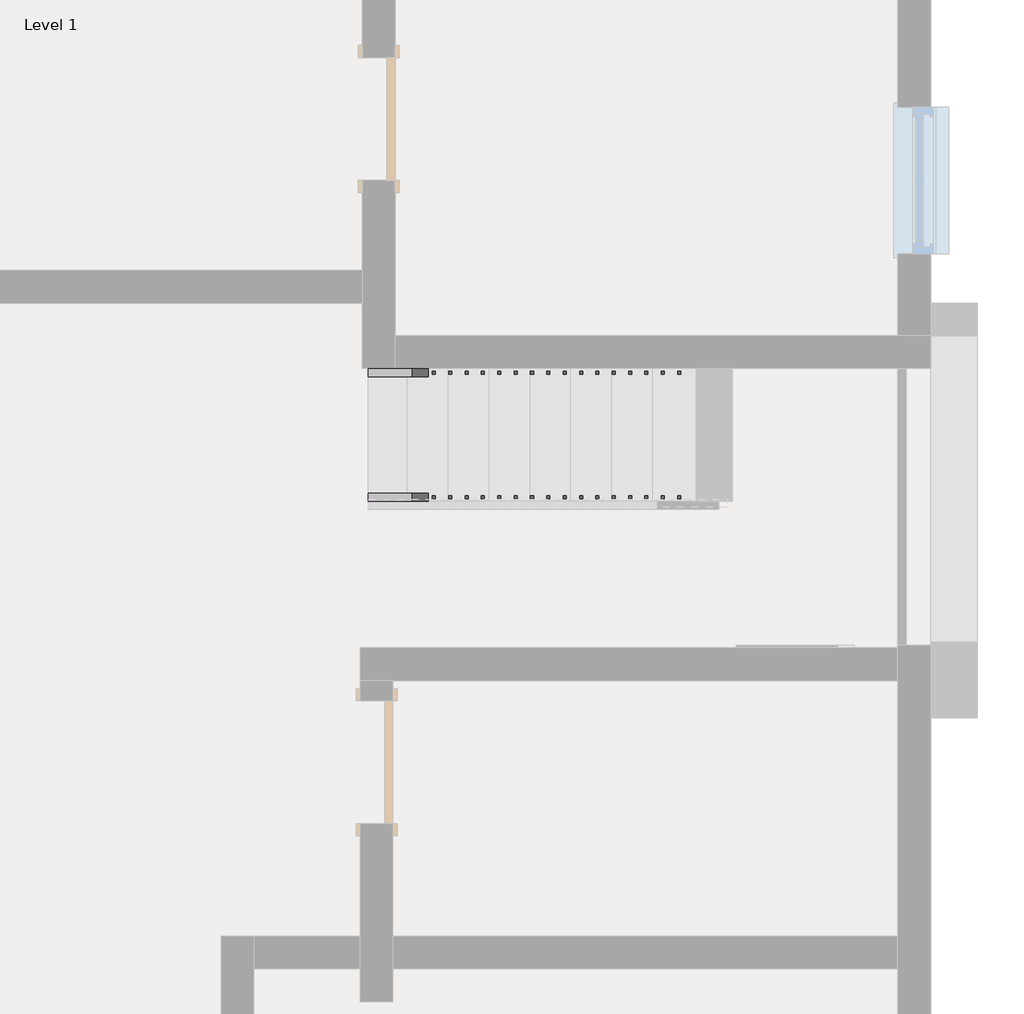
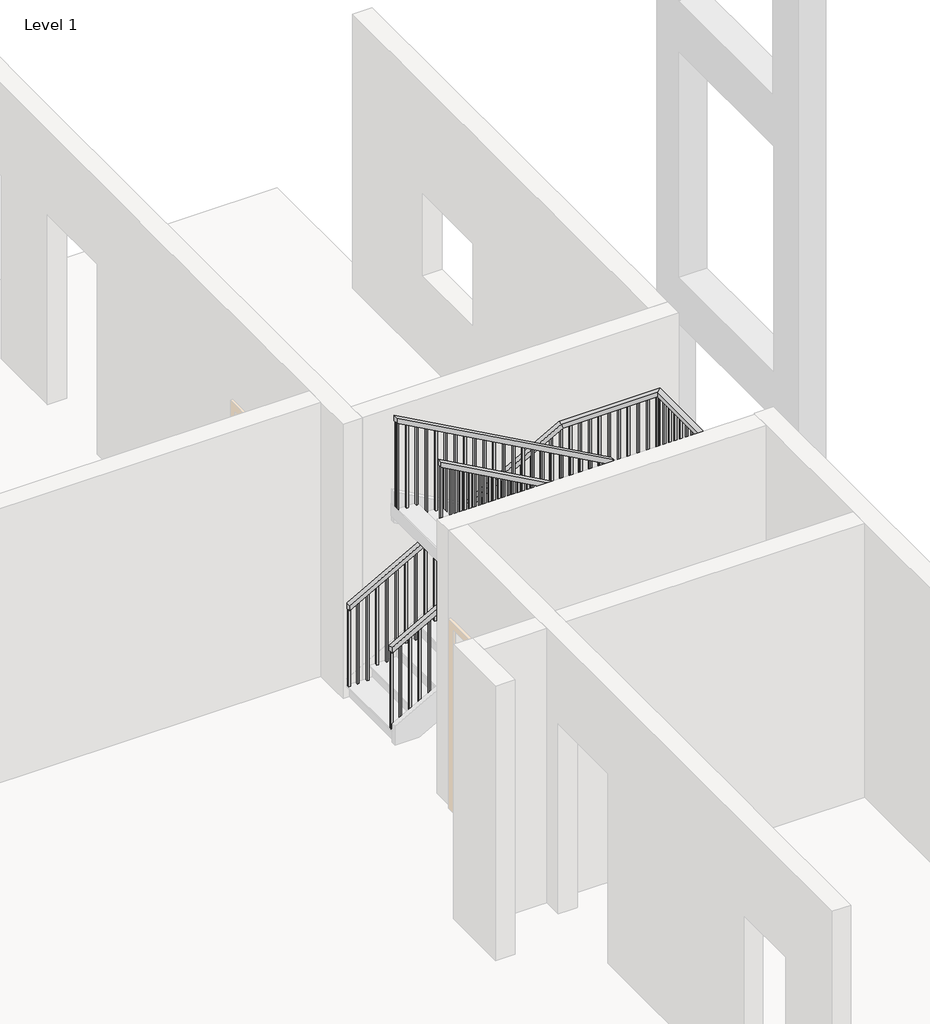
# One storey, part 3 of 4: 2 railings.
"""IFC4 building model written with IfcOpenShell, lengths in millimetres."""

from ifc_helpers import new_model, si_unit, frame, origin, place, context, project, spatial, polyline, outline, extrude, faceted_brep, element, save

model = new_model("IFC4")

# Units and contexts
model_context = context("Model", 3, world=origin())
ifc_project = project(units=[si_unit("LENGTHUNIT", "METRE", prefix="MILLI")], contexts=[model_context])

# Site, building, storey
site = spatial("IfcSite", under=ifc_project)
building = spatial("IfcBuilding", under=site)
storey = spatial("IfcBuildingStorey", under=building, Name="Level 1", Elevation=0.0)

# Railings
placement = place(None, origin())
element("IfcRailing", 1, ObjectType="Handrail - Rectangular", at=placement, inside=storey, context=model_context, shape_type="SolidModel", body=[
    faceted_brep([(1537.1941283, 231.7547293, 1051.56), (1537.1941283, 231.7547293, 993.4879132), (1537.1941283, 180.9547293, 993.4879132), (1537.1941283, 180.9547293, 1051.56), (3765.8648053, 231.7547293, 2286.0), (3765.8648053, 180.9547293, 2286.0), (3765.8648053, 180.9547293, 2227.9279132), (3765.8648053, 231.7547293, 2227.9279132)], [[[0, 1, 2, 3]], [[4, 5, 6, 7]], [[1, 0, 4, 7]], [[2, 1, 7, 6]], [[3, 2, 6, 5]], [[0, 3, 5, 4]]]),
    faceted_brep([(3816.6648053, 231.7547293, 2286.0), (3816.6648053, 231.7547293, 2235.2), (3765.8648053, 231.7547293, 2235.2), (3765.8648053, 231.7547293, 2286.0), (3816.6648053, 142.8547293, 2286.0), (3765.8648053, 142.8547293, 2286.0), (3765.8648053, 92.0547293, 2235.2), (3816.6648053, 92.0547293, 2235.2)], [[[0, 1, 2, 3]], [[4, 5, 6, 7]], [[1, 0, 4, 7]], [[2, 1, 7, 6]], [[3, 2, 6, 5]], [[0, 3, 5, 4]]]),
    faceted_brep([(3816.6648053, 142.8547293, 2286.0), (3816.6648053, 92.0547293, 2235.2), (3765.8648053, 92.0547293, 2235.2), (3765.8648053, 142.8547293, 2286.0), (3816.6648053, 142.8547293, 2395.0223516), (3765.8648053, 142.8547293, 2365.0879132), (3765.8648053, 92.0547293, 2365.0879132), (3816.6648053, 92.0547293, 2395.0223516)], [[[0, 1, 2, 3]], [[4, 5, 6, 7]], [[1, 0, 4, 7]], [[2, 1, 7, 6]], [[3, 2, 6, 5]], [[0, 3, 5, 4]]]),
    faceted_brep([(3816.6648053, 92.0547293, 2395.0223516), (3765.8648053, 92.0547293, 2365.0879132), (3765.8648053, 142.8547293, 2365.0879132), (3816.6648053, 142.8547293, 2395.0223516), (1537.1941283, 92.0547293, 3657.6), (1537.1941283, 142.8547293, 3657.6), (1537.1941283, 142.8547293, 3599.5279132), (1537.1941283, 92.0547293, 3599.5279132)], [[[0, 1, 2, 3]], [[4, 5, 6, 7]], [[1, 0, 4, 7]], [[2, 1, 7, 6]], [[3, 2, 6, 5]], [[0, 3, 5, 4]]]),
    extrude(outline(polyline([(3583.7556667, 1565.5898053), (3594.3072849, 1546.5398053), (2606.04, 1546.5398053), (2606.04, 1565.5898053), (3583.7556667, 1565.5898053)])), frame((0.0, 107.9297293, 0.0), z_axis=(0.0, 1.0, 0.0), x_axis=(0.0, 0.0, 1.0)), (0.0, 0.0, 1.0), 19.05),
    extrude(outline(polyline([(3527.4803699, 1667.1898053), (3538.031988, 1648.1398053), (2606.04, 1648.1398053), (2606.04, 1667.1898053), (3527.4803699, 1667.1898053)])), frame((0.0, 107.9297293, 0.0), z_axis=(0.0, 1.0, 0.0), x_axis=(0.0, 0.0, 1.0)), (0.0, 0.0, 1.0), 19.05),
    extrude(outline(polyline([(3471.1609284, 1768.7898053), (3481.7125466, 1749.7398053), (2606.04, 1749.7398053), (2606.04, 1768.7898053), (3471.1609284, 1768.7898053)])), frame((0.0, 107.9297293, 0.0), z_axis=(0.0, 1.0, 0.0), x_axis=(0.0, 0.0, 1.0)), (0.0, 0.0, 1.0), 19.05),
    extrude(outline(polyline([(3414.9297761, 1870.3898053), (3425.4813943, 1851.3398053), (2468.88, 1851.3398053), (2468.88, 1870.3898053), (3414.9297761, 1870.3898053)])), frame((0.0, 107.9297293, 0.0), z_axis=(0.0, 1.0, 0.0), x_axis=(0.0, 0.0, 1.0)), (0.0, 0.0, 1.0), 19.05),
    extrude(outline(polyline([(3358.6544792, 1971.9898053), (3369.2060974, 1952.9398053), (2468.88, 1952.9398053), (2468.88, 1971.9898053), (3358.6544792, 1971.9898053)])), frame((0.0, 107.9297293, 0.0), z_axis=(0.0, 1.0, 0.0), x_axis=(0.0, 0.0, 1.0)), (0.0, 0.0, 1.0), 19.05),
    extrude(outline(polyline([(3302.3791823, 2073.5898053), (3312.9308005, 2054.5398053), (2331.72, 2054.5398053), (2331.72, 2073.5898053), (3302.3791823, 2073.5898053)])), frame((0.0, 107.9297293, 0.0), z_axis=(0.0, 1.0, 0.0), x_axis=(0.0, 0.0, 1.0)), (0.0, 0.0, 1.0), 19.05),
    extrude(outline(polyline([(3246.1038855, 2175.1898053), (3256.6555036, 2156.1398053), (2331.72, 2156.1398053), (2331.72, 2175.1898053), (3246.1038855, 2175.1898053)])), frame((0.0, 107.9297293, 0.0), z_axis=(0.0, 1.0, 0.0), x_axis=(0.0, 0.0, 1.0)), (0.0, 0.0, 1.0), 19.05),
    extrude(outline(polyline([(3189.8285886, 2276.7898053), (3200.3802067, 2257.7398053), (2331.72, 2257.7398053), (2331.72, 2276.7898053), (3189.8285886, 2276.7898053)])), frame((0.0, 107.9297293, 0.0), z_axis=(0.0, 1.0, 0.0), x_axis=(0.0, 0.0, 1.0)), (0.0, 0.0, 1.0), 19.05),
    extrude(outline(polyline([(3133.5532917, 2378.3898053), (3144.1049099, 2359.3398053), (2194.56, 2359.3398053), (2194.56, 2378.3898053), (3133.5532917, 2378.3898053)])), frame((0.0, 107.9297293, 0.0), z_axis=(0.0, 1.0, 0.0), x_axis=(0.0, 0.0, 1.0)), (0.0, 0.0, 1.0), 19.05),
    extrude(outline(polyline([(3077.2779948, 2479.9898053), (3087.829613, 2460.9398053), (2194.56, 2460.9398053), (2194.56, 2479.9898053), (3077.2779948, 2479.9898053)])), frame((0.0, 107.9297293, 0.0), z_axis=(0.0, 1.0, 0.0), x_axis=(0.0, 0.0, 1.0)), (0.0, 0.0, 1.0), 19.05),
    extrude(outline(polyline([(3021.0026979, 2581.5898053), (3031.5543161, 2562.5398053), (2057.4, 2562.5398053), (2057.4, 2581.5898053), (3021.0026979, 2581.5898053)])), frame((0.0, 107.9297293, 0.0), z_axis=(0.0, 1.0, 0.0), x_axis=(0.0, 0.0, 1.0)), (0.0, 0.0, 1.0), 19.05),
    extrude(outline(polyline([(2964.727401, 2683.1898053), (2975.2790192, 2664.1398053), (2057.4, 2664.1398053), (2057.4, 2683.1898053), (2964.727401, 2683.1898053)])), frame((0.0, 107.9297293, 0.0), z_axis=(0.0, 1.0, 0.0), x_axis=(0.0, 0.0, 1.0)), (0.0, 0.0, 1.0), 19.05),
    extrude(outline(polyline([(2908.4962488, 2784.7898053), (2919.0478669, 2765.7398053), (2057.4, 2765.7398053), (2057.4, 2784.7898053), (2908.4962488, 2784.7898053)])), frame((0.0, 107.9297293, 0.0), z_axis=(0.0, 1.0, 0.0), x_axis=(0.0, 0.0, 1.0)), (0.0, 0.0, 1.0), 19.05),
    extrude(outline(polyline([(2852.2209519, 2886.3898053), (2862.77257, 2867.3398053), (1920.24, 2867.3398053), (1920.24, 2886.3898053), (2852.2209519, 2886.3898053)])), frame((0.0, 107.9297293, 0.0), z_axis=(0.0, 1.0, 0.0), x_axis=(0.0, 0.0, 1.0)), (0.0, 0.0, 1.0), 19.05),
    extrude(outline(polyline([(2795.945655, 2987.9898053), (2806.4972732, 2968.9398053), (1920.24, 2968.9398053), (1920.24, 2987.9898053), (2795.945655, 2987.9898053)])), frame((0.0, 107.9297293, 0.0), z_axis=(0.0, 1.0, 0.0), x_axis=(0.0, 0.0, 1.0)), (0.0, 0.0, 1.0), 19.05),
    extrude(outline(polyline([(2739.6703581, 3089.5898053), (2750.2219763, 3070.5398053), (1783.08, 3070.5398053), (1783.08, 3089.5898053), (2739.6703581, 3089.5898053)])), frame((0.0, 107.9297293, 0.0), z_axis=(0.0, 1.0, 0.0), x_axis=(0.0, 0.0, 1.0)), (0.0, 0.0, 1.0), 19.05),
    extrude(outline(polyline([(2683.3950612, 3191.1898053), (2693.9466794, 3172.1398053), (1783.08, 3172.1398053), (1783.08, 3191.1898053), (2683.3950612, 3191.1898053)])), frame((0.0, 107.9297293, 0.0), z_axis=(0.0, 1.0, 0.0), x_axis=(0.0, 0.0, 1.0)), (0.0, 0.0, 1.0), 19.05),
    extrude(outline(polyline([(2627.1197643, 3292.7898053), (2637.6713825, 3273.7398053), (1783.08, 3273.7398053), (1783.08, 3292.7898053), (2627.1197643, 3292.7898053)])), frame((0.0, 107.9297293, 0.0), z_axis=(0.0, 1.0, 0.0), x_axis=(0.0, 0.0, 1.0)), (0.0, 0.0, 1.0), 19.05),
    extrude(outline(polyline([(2570.8444675, 3394.3898053), (2581.3960856, 3375.3398053), (1645.92, 3375.3398053), (1645.92, 3394.3898053), (2570.8444675, 3394.3898053)])), frame((0.0, 107.9297293, 0.0), z_axis=(0.0, 1.0, 0.0), x_axis=(0.0, 0.0, 1.0)), (0.0, 0.0, 1.0), 19.05),
    extrude(outline(polyline([(2514.5691706, 3495.9898053), (2525.1207888, 3476.9398053), (1645.92, 3476.9398053), (1645.92, 3495.9898053), (2514.5691706, 3495.9898053)])), frame((0.0, 107.9297293, 0.0), z_axis=(0.0, 1.0, 0.0), x_axis=(0.0, 0.0, 1.0)), (0.0, 0.0, 1.0), 19.05),
    extrude(outline(polyline([(2458.2938737, 3597.5898053), (2468.8454919, 3578.5398053), (1508.76, 3578.5398053), (1508.76, 3597.5898053), (2458.2938737, 3597.5898053)])), frame((0.0, 107.9297293, 0.0), z_axis=(0.0, 1.0, 0.0), x_axis=(0.0, 0.0, 1.0)), (0.0, 0.0, 1.0), 19.05),
    extrude(outline(polyline([(2402.0185768, 3699.1898053), (2412.570195, 3680.1398053), (1508.76, 3680.1398053), (1508.76, 3699.1898053), (2402.0185768, 3699.1898053)])), frame((0.0, 107.9297293, 0.0), z_axis=(0.0, 1.0, 0.0), x_axis=(0.0, 0.0, 1.0)), (0.0, 0.0, 1.0), 19.05),
    extrude(outline(polyline([(2236.8202537, 3781.9191283), (2226.2686355, 3762.8691283), (1371.6, 3762.8691283), (1371.6, 3781.9191283), (2236.8202537, 3781.9191283)])), frame((0.0, 196.8297293, 0.0), z_axis=(0.0, 1.0, 0.0), x_axis=(0.0, 0.0, 1.0)), (0.0, 0.0, 1.0), 19.05),
    extrude(outline(polyline([(2180.5449568, 3680.3191283), (2169.9933387, 3661.2691283), (1234.44, 3661.2691283), (1234.44, 3680.3191283), (2180.5449568, 3680.3191283)])), frame((0.0, 196.8297293, 0.0), z_axis=(0.0, 1.0, 0.0), x_axis=(0.0, 0.0, 1.0)), (0.0, 0.0, 1.0), 19.05),
    extrude(outline(polyline([(2124.26966, 3578.7191283), (2113.7180418, 3559.6691283), (1234.44, 3559.6691283), (1234.44, 3578.7191283), (2124.26966, 3578.7191283)])), frame((0.0, 196.8297293, 0.0), z_axis=(0.0, 1.0, 0.0), x_axis=(0.0, 0.0, 1.0)), (0.0, 0.0, 1.0), 19.05),
    extrude(outline(polyline([(2067.9943631, 3477.1191283), (2057.4427449, 3458.0691283), (1097.28, 3458.0691283), (1097.28, 3477.1191283), (2067.9943631, 3477.1191283)])), frame((0.0, 196.8297293, 0.0), z_axis=(0.0, 1.0, 0.0), x_axis=(0.0, 0.0, 1.0)), (0.0, 0.0, 1.0), 19.05),
    extrude(outline(polyline([(2011.7190662, 3375.5191283), (2001.167448, 3356.4691283), (1097.28, 3356.4691283), (1097.28, 3375.5191283), (2011.7190662, 3375.5191283)])), frame((0.0, 196.8297293, 0.0), z_axis=(0.0, 1.0, 0.0), x_axis=(0.0, 0.0, 1.0)), (0.0, 0.0, 1.0), 19.05),
    extrude(outline(polyline([(1955.4437693, 3273.9191283), (1944.8921511, 3254.8691283), (960.12, 3254.8691283), (960.12, 3273.9191283), (1955.4437693, 3273.9191283)])), frame((0.0, 196.8297293, 0.0), z_axis=(0.0, 1.0, 0.0), x_axis=(0.0, 0.0, 1.0)), (0.0, 0.0, 1.0), 19.05),
    extrude(outline(polyline([(1899.1684724, 3172.3191283), (1888.6168543, 3153.2691283), (960.12, 3153.2691283), (960.12, 3172.3191283), (1899.1684724, 3172.3191283)])), frame((0.0, 196.8297293, 0.0), z_axis=(0.0, 1.0, 0.0), x_axis=(0.0, 0.0, 1.0)), (0.0, 0.0, 1.0), 19.05),
    extrude(outline(polyline([(1842.8931755, 3070.7191283), (1832.3415574, 3051.6691283), (960.12, 3051.6691283), (960.12, 3070.7191283), (1842.8931755, 3070.7191283)])), frame((0.0, 196.8297293, 0.0), z_axis=(0.0, 1.0, 0.0), x_axis=(0.0, 0.0, 1.0)), (0.0, 0.0, 1.0), 19.05),
    extrude(outline(polyline([(1786.6178787, 2969.1191283), (1776.0662605, 2950.0691283), (822.96, 2950.0691283), (822.96, 2969.1191283), (1786.6178787, 2969.1191283)])), frame((0.0, 196.8297293, 0.0), z_axis=(0.0, 1.0, 0.0), x_axis=(0.0, 0.0, 1.0)), (0.0, 0.0, 1.0), 19.05),
    extrude(outline(polyline([(1730.3425818, 2867.5191283), (1719.7909636, 2848.4691283), (822.96, 2848.4691283), (822.96, 2867.5191283), (1730.3425818, 2867.5191283)])), frame((0.0, 196.8297293, 0.0), z_axis=(0.0, 1.0, 0.0), x_axis=(0.0, 0.0, 1.0)), (0.0, 0.0, 1.0), 19.05),
    extrude(outline(polyline([(1674.0672849, 2765.9191283), (1663.5156667, 2746.8691283), (685.8, 2746.8691283), (685.8, 2765.9191283), (1674.0672849, 2765.9191283)])), frame((0.0, 196.8297293, 0.0), z_axis=(0.0, 1.0, 0.0), x_axis=(0.0, 0.0, 1.0)), (0.0, 0.0, 1.0), 19.05),
    extrude(outline(polyline([(1617.791988, 2664.3191283), (1607.2403699, 2645.2691283), (685.8, 2645.2691283), (685.8, 2664.3191283), (1617.791988, 2664.3191283)])), frame((0.0, 196.8297293, 0.0), z_axis=(0.0, 1.0, 0.0), x_axis=(0.0, 0.0, 1.0)), (0.0, 0.0, 1.0), 19.05),
    extrude(outline(polyline([(1561.4725466, 2562.7191283), (1550.9209284, 2543.6691283), (685.8, 2543.6691283), (685.8, 2562.7191283), (1561.4725466, 2562.7191283)])), frame((0.0, 196.8297293, 0.0), z_axis=(0.0, 1.0, 0.0), x_axis=(0.0, 0.0, 1.0)), (0.0, 0.0, 1.0), 19.05),
    extrude(outline(polyline([(1505.2413943, 2461.1191283), (1494.6897761, 2442.0691283), (548.64, 2442.0691283), (548.64, 2461.1191283), (1505.2413943, 2461.1191283)])), frame((0.0, 196.8297293, 0.0), z_axis=(0.0, 1.0, 0.0), x_axis=(0.0, 0.0, 1.0)), (0.0, 0.0, 1.0), 19.05),
    extrude(outline(polyline([(1448.9660974, 2359.5191283), (1438.4144792, 2340.4691283), (548.64, 2340.4691283), (548.64, 2359.5191283), (1448.9660974, 2359.5191283)])), frame((0.0, 196.8297293, 0.0), z_axis=(0.0, 1.0, 0.0), x_axis=(0.0, 0.0, 1.0)), (0.0, 0.0, 1.0), 19.05),
    extrude(outline(polyline([(1392.6908005, 2257.9191283), (1382.1391823, 2238.8691283), (411.48, 2238.8691283), (411.48, 2257.9191283), (1392.6908005, 2257.9191283)])), frame((0.0, 196.8297293, 0.0), z_axis=(0.0, 1.0, 0.0), x_axis=(0.0, 0.0, 1.0)), (0.0, 0.0, 1.0), 19.05),
    extrude(outline(polyline([(1336.4155036, 2156.3191283), (1325.8638855, 2137.2691283), (411.48, 2137.2691283), (411.48, 2156.3191283), (1336.4155036, 2156.3191283)])), frame((0.0, 196.8297293, 0.0), z_axis=(0.0, 1.0, 0.0), x_axis=(0.0, 0.0, 1.0)), (0.0, 0.0, 1.0), 19.05),
    extrude(outline(polyline([(1280.1402067, 2054.7191283), (1269.5885886, 2035.6691283), (411.48, 2035.6691283), (411.48, 2054.7191283), (1280.1402067, 2054.7191283)])), frame((0.0, 196.8297293, 0.0), z_axis=(0.0, 1.0, 0.0), x_axis=(0.0, 0.0, 1.0)), (0.0, 0.0, 1.0), 19.05),
    extrude(outline(polyline([(1223.8649099, 1953.1191283), (1213.3132917, 1934.0691283), (274.32, 1934.0691283), (274.32, 1953.1191283), (1223.8649099, 1953.1191283)])), frame((0.0, 196.8297293, 0.0), z_axis=(0.0, 1.0, 0.0), x_axis=(0.0, 0.0, 1.0)), (0.0, 0.0, 1.0), 19.05),
    extrude(outline(polyline([(1167.589613, 1851.5191283), (1157.0379948, 1832.4691283), (274.32, 1832.4691283), (274.32, 1851.5191283), (1167.589613, 1851.5191283)])), frame((0.0, 196.8297293, 0.0), z_axis=(0.0, 1.0, 0.0), x_axis=(0.0, 0.0, 1.0)), (0.0, 0.0, 1.0), 19.05),
    extrude(outline(polyline([(1111.3143161, 1749.9191283), (1100.7626979, 1730.8691283), (137.16, 1730.8691283), (137.16, 1749.9191283), (1111.3143161, 1749.9191283)])), frame((0.0, 196.8297293, 0.0), z_axis=(0.0, 1.0, 0.0), x_axis=(0.0, 0.0, 1.0)), (0.0, 0.0, 1.0), 19.05),
    extrude(outline(polyline([(1055.0390192, 1648.3191283), (1044.487401, 1629.2691283), (137.16, 1629.2691283), (137.16, 1648.3191283), (1055.0390192, 1648.3191283)])), frame((0.0, 196.8297293, 0.0), z_axis=(0.0, 1.0, 0.0), x_axis=(0.0, 0.0, 1.0)), (0.0, 0.0, 1.0), 19.05),
    extrude(outline(polyline([(3781.7398053, 126.9797293), (3800.7898053, 126.9797293), (3800.7898053, 107.9297293), (3781.7398053, 107.9297293), (3781.7398053, 126.9797293)])), frame((0.0, 0.0, 1371.6), z_axis=(0.0, 0.0, 1.0), x_axis=(1.0, 0.0, 0.0)), (0.0, 0.0, 1.0), 863.6),
    extrude(outline(polyline([(2247.2725466, 3800.7898053), (2236.7209284, 3781.7398053), (1371.6, 3781.7398053), (1371.6, 3800.7898053), (2247.2725466, 3800.7898053)])), frame((0.0, 196.8297293, 0.0), z_axis=(0.0, 1.0, 0.0), x_axis=(0.0, 0.0, 1.0)), (0.0, 0.0, 1.0), 19.05),
    extrude(outline(polyline([(3588.9762951, 1556.2441283), (3599.5279132, 1537.1941283), (2606.04, 1537.1941283), (2606.04, 1556.2441283), (3588.9762951, 1556.2441283)])), frame((0.0, 107.9297293, 0.0), z_axis=(0.0, 1.0, 0.0), x_axis=(0.0, 0.0, 1.0)), (0.0, 0.0, 1.0), 19.05),
    extrude(outline(polyline([(1004.0395314, 1556.2441283), (993.4879132, 1537.1941283), (137.16, 1537.1941283), (137.16, 1556.2441283), (1004.0395314, 1556.2441283)])), frame((0.0, 196.8297293, 0.0), z_axis=(0.0, 1.0, 0.0), x_axis=(0.0, 0.0, 1.0)), (0.0, 0.0, 1.0), 19.05),
])
element("IfcRailing", 2, ObjectType="Handrail - Rectangular", at=placement, inside=storey, context=model_context, shape_type="SolidModel", body=[
    faceted_brep([(1537.1941283, 1006.4547293, 1051.56), (1537.1941283, 1006.4547293, 993.4879132), (1537.1941283, 955.6547293, 993.4879132), (1537.1941283, 955.6547293, 1051.56), (3765.8648053, 1006.4547293, 2286.0), (3778.9939056, 1006.4547293, 2235.2), (3778.9939056, 955.6547293, 2235.2), (3765.8648053, 955.6547293, 2286.0), (4826.4941283, 1006.4547293, 2286.0), (4826.4941283, 1006.4547293, 2235.2), (4775.6941283, 955.6547293, 2235.2), (4775.6941283, 955.6547293, 2286.0), (4826.4941283, -714.2964201, 2286.0), (4826.4941283, -714.2964201, 2235.2), (4775.6941283, -663.4964201, 2235.2), (4775.6941283, -663.4964201, 2286.0), (4013.4948805, -714.2964201, 2286.0), (4000.3657803, -714.2964201, 2235.2), (4000.3657803, -663.4964201, 2235.2), (4013.4948805, -663.4964201, 2286.0), (1537.1941283, -714.2964201, 3657.6), (1537.1941283, -663.4964201, 3657.6), (1537.1941283, -663.4964201, 3599.5279132), (1537.1941283, -714.2964201, 3599.5279132)], [[[0, 1, 2, 3]], [[1, 0, 4, 5]], [[2, 1, 5, 6]], [[3, 2, 6, 7]], [[0, 3, 7, 4]], [[5, 4, 8, 9]], [[6, 5, 9, 10]], [[7, 6, 10, 11]], [[4, 7, 11, 8]], [[9, 8, 12, 13]], [[10, 9, 13, 14]], [[11, 10, 14, 15]], [[8, 11, 15, 12]], [[13, 12, 16, 17]], [[14, 13, 17, 18]], [[15, 14, 18, 19]], [[12, 15, 19, 16]], [[20, 21, 22, 23]], [[17, 16, 20, 23]], [[18, 17, 23, 22]], [[19, 18, 22, 21]], [[16, 19, 21, 20]]]),
    extrude(outline(polyline([(3597.7693102, 1540.3691283), (2606.04, 1540.3691283), (2606.04, 1559.4191283), (3587.2176921, 1559.4191283), (3597.7693102, 1540.3691283)])), frame((0.0, -698.4214201, 0.0), z_axis=(0.0, 1.0, 0.0), x_axis=(0.0, 0.0, 1.0)), (0.0, 0.0, 1.0), 19.05),
    extrude(outline(polyline([(3541.4940133, 1641.9691283), (2606.04, 1641.9691283), (2606.04, 1661.0191283), (3530.9423952, 1661.0191283), (3541.4940133, 1641.9691283)])), frame((0.0, -698.4214201, 0.0), z_axis=(0.0, 1.0, 0.0), x_axis=(0.0, 0.0, 1.0)), (0.0, 0.0, 1.0), 19.05),
    extrude(outline(polyline([(3485.2187165, 1743.5691283), (2606.04, 1743.5691283), (2606.04, 1762.6191283), (3474.6670983, 1762.6191283), (3485.2187165, 1743.5691283)])), frame((0.0, -698.4214201, 0.0), z_axis=(0.0, 1.0, 0.0), x_axis=(0.0, 0.0, 1.0)), (0.0, 0.0, 1.0), 19.05),
    extrude(outline(polyline([(3428.9434196, 1845.1691283), (2468.88, 1845.1691283), (2468.88, 1864.2191283), (3418.3918014, 1864.2191283), (3428.9434196, 1845.1691283)])), frame((0.0, -698.4214201, 0.0), z_axis=(0.0, 1.0, 0.0), x_axis=(0.0, 0.0, 1.0)), (0.0, 0.0, 1.0), 19.05),
    extrude(outline(polyline([(3372.6681227, 1946.7691283), (2468.88, 1946.7691283), (2468.88, 1965.8191283), (3362.1165045, 1965.8191283), (3372.6681227, 1946.7691283)])), frame((0.0, -698.4214201, 0.0), z_axis=(0.0, 1.0, 0.0), x_axis=(0.0, 0.0, 1.0)), (0.0, 0.0, 1.0), 19.05),
    extrude(outline(polyline([(3316.3928258, 2048.3691283), (2331.72, 2048.3691283), (2331.72, 2067.4191283), (3305.8412076, 2067.4191283), (3316.3928258, 2048.3691283)])), frame((0.0, -698.4214201, 0.0), z_axis=(0.0, 1.0, 0.0), x_axis=(0.0, 0.0, 1.0)), (0.0, 0.0, 1.0), 19.05),
    extrude(outline(polyline([(3260.1175289, 2149.9691283), (2331.72, 2149.9691283), (2331.72, 2169.0191283), (3249.5659108, 2169.0191283), (3260.1175289, 2149.9691283)])), frame((0.0, -698.4214201, 0.0), z_axis=(0.0, 1.0, 0.0), x_axis=(0.0, 0.0, 1.0)), (0.0, 0.0, 1.0), 19.05),
    extrude(outline(polyline([(3203.8422321, 2251.5691283), (2331.72, 2251.5691283), (2331.72, 2270.6191283), (3193.2906139, 2270.6191283), (3203.8422321, 2251.5691283)])), frame((0.0, -698.4214201, 0.0), z_axis=(0.0, 1.0, 0.0), x_axis=(0.0, 0.0, 1.0)), (0.0, 0.0, 1.0), 19.05),
    extrude(outline(polyline([(3147.5669352, 2353.1691283), (2194.56, 2353.1691283), (2194.56, 2372.2191283), (3137.015317, 2372.2191283), (3147.5669352, 2353.1691283)])), frame((0.0, -698.4214201, 0.0), z_axis=(0.0, 1.0, 0.0), x_axis=(0.0, 0.0, 1.0)), (0.0, 0.0, 1.0), 19.05),
    extrude(outline(polyline([(3091.2916383, 2454.7691283), (2194.56, 2454.7691283), (2194.56, 2473.8191283), (3080.7400201, 2473.8191283), (3091.2916383, 2454.7691283)])), frame((0.0, -698.4214201, 0.0), z_axis=(0.0, 1.0, 0.0), x_axis=(0.0, 0.0, 1.0)), (0.0, 0.0, 1.0), 19.05),
    extrude(outline(polyline([(3035.0163414, 2556.3691283), (2057.4, 2556.3691283), (2057.4, 2575.4191283), (3024.4647232, 2575.4191283), (3035.0163414, 2556.3691283)])), frame((0.0, -698.4214201, 0.0), z_axis=(0.0, 1.0, 0.0), x_axis=(0.0, 0.0, 1.0)), (0.0, 0.0, 1.0), 19.05),
    extrude(outline(polyline([(2978.7410445, 2657.9691283), (2057.4, 2657.9691283), (2057.4, 2677.0191283), (2968.1894264, 2677.0191283), (2978.7410445, 2657.9691283)])), frame((0.0, -698.4214201, 0.0), z_axis=(0.0, 1.0, 0.0), x_axis=(0.0, 0.0, 1.0)), (0.0, 0.0, 1.0), 19.05),
    extrude(outline(polyline([(2922.4657476, 2759.5691283), (2057.4, 2759.5691283), (2057.4, 2778.6191283), (2911.9141295, 2778.6191283), (2922.4657476, 2759.5691283)])), frame((0.0, -698.4214201, 0.0), z_axis=(0.0, 1.0, 0.0), x_axis=(0.0, 0.0, 1.0)), (0.0, 0.0, 1.0), 19.05),
    extrude(outline(polyline([(2866.3449568, 2861.1691283), (1920.24, 2861.1691283), (1920.24, 2880.2191283), (2855.7933387, 2880.2191283), (2866.3449568, 2861.1691283)])), frame((0.0, -698.4214201, 0.0), z_axis=(0.0, 1.0, 0.0), x_axis=(0.0, 0.0, 1.0)), (0.0, 0.0, 1.0), 19.05),
    extrude(outline(polyline([(2810.06966, 2962.7691283), (1920.24, 2962.7691283), (1920.24, 2981.8191283), (2799.5180418, 2981.8191283), (2810.06966, 2962.7691283)])), frame((0.0, -698.4214201, 0.0), z_axis=(0.0, 1.0, 0.0), x_axis=(0.0, 0.0, 1.0)), (0.0, 0.0, 1.0), 19.05),
    extrude(outline(polyline([(2753.7943631, 3064.3691283), (1783.08, 3064.3691283), (1783.08, 3083.4191283), (2743.2427449, 3083.4191283), (2753.7943631, 3064.3691283)])), frame((0.0, -698.4214201, 0.0), z_axis=(0.0, 1.0, 0.0), x_axis=(0.0, 0.0, 1.0)), (0.0, 0.0, 1.0), 19.05),
    extrude(outline(polyline([(2697.5190662, 3165.9691283), (1783.08, 3165.9691283), (1783.08, 3185.0191283), (2686.967448, 3185.0191283), (2697.5190662, 3165.9691283)])), frame((0.0, -698.4214201, 0.0), z_axis=(0.0, 1.0, 0.0), x_axis=(0.0, 0.0, 1.0)), (0.0, 0.0, 1.0), 19.05),
    extrude(outline(polyline([(2641.0892632, 3267.5691283), (1783.08, 3267.5691283), (1783.08, 3286.6191283), (2630.5376451, 3286.6191283), (2641.0892632, 3267.5691283)])), frame((0.0, -698.4214201, 0.0), z_axis=(0.0, 1.0, 0.0), x_axis=(0.0, 0.0, 1.0)), (0.0, 0.0, 1.0), 19.05),
    extrude(outline(polyline([(2584.9684724, 3369.1691283), (1645.92, 3369.1691283), (1645.92, 3388.2191283), (2574.4168543, 3388.2191283), (2584.9684724, 3369.1691283)])), frame((0.0, -698.4214201, 0.0), z_axis=(0.0, 1.0, 0.0), x_axis=(0.0, 0.0, 1.0)), (0.0, 0.0, 1.0), 19.05),
    extrude(outline(polyline([(2528.6931755, 3470.7691283), (1645.92, 3470.7691283), (1645.92, 3489.8191283), (2518.1415574, 3489.8191283), (2528.6931755, 3470.7691283)])), frame((0.0, -698.4214201, 0.0), z_axis=(0.0, 1.0, 0.0), x_axis=(0.0, 0.0, 1.0)), (0.0, 0.0, 1.0), 19.05),
    extrude(outline(polyline([(2472.4178787, 3572.3691283), (1508.76, 3572.3691283), (1508.76, 3591.4191283), (2461.8662605, 3591.4191283), (2472.4178787, 3572.3691283)])), frame((0.0, -698.4214201, 0.0), z_axis=(0.0, 1.0, 0.0), x_axis=(0.0, 0.0, 1.0)), (0.0, 0.0, 1.0), 19.05),
    extrude(outline(polyline([(2416.1425818, 3673.9691283), (1508.76, 3673.9691283), (1508.76, 3693.0191283), (2405.5909636, 3693.0191283), (2416.1425818, 3673.9691283)])), frame((0.0, -698.4214201, 0.0), z_axis=(0.0, 1.0, 0.0), x_axis=(0.0, 0.0, 1.0)), (0.0, 0.0, 1.0), 19.05),
    extrude(outline(polyline([(2359.8672849, 3775.5691283), (1371.6, 3775.5691283), (1371.6, 3794.6191283), (2349.3156667, 3794.6191283), (2359.8672849, 3775.5691283)])), frame((0.0, -698.4214201, 0.0), z_axis=(0.0, 1.0, 0.0), x_axis=(0.0, 0.0, 1.0)), (0.0, 0.0, 1.0), 19.05),
    extrude(outline(polyline([(2303.591988, 3877.1691283), (1371.6, 3877.1691283), (1371.6, 3896.2191283), (2293.0403699, 3896.2191283), (2303.591988, 3877.1691283)])), frame((0.0, -698.4214201, 0.0), z_axis=(0.0, 1.0, 0.0), x_axis=(0.0, 0.0, 1.0)), (0.0, 0.0, 1.0), 19.05),
    extrude(outline(polyline([(2247.3166911, 3978.7691283), (1371.6, 3978.7691283), (1371.6, 3997.8191283), (2236.765073, 3997.8191283), (2247.3166911, 3978.7691283)])), frame((0.0, -698.4214201, 0.0), z_axis=(0.0, 1.0, 0.0), x_axis=(0.0, 0.0, 1.0)), (0.0, 0.0, 1.0), 19.05),
    extrude(outline(polyline([(4099.4191283, -698.4214201), (4080.3691283, -698.4214201), (4080.3691283, -679.3714201), (4099.4191283, -679.3714201), (4099.4191283, -698.4214201)])), frame((0.0, 0.0, 1371.6), z_axis=(0.0, 0.0, 1.0), x_axis=(1.0, 0.0, 0.0)), (0.0, 0.0, 1.0), 863.6),
    extrude(outline(polyline([(4201.0191283, -698.4214201), (4181.9691283, -698.4214201), (4181.9691283, -679.3714201), (4201.0191283, -679.3714201), (4201.0191283, -698.4214201)])), frame((0.0, 0.0, 1371.6), z_axis=(0.0, 0.0, 1.0), x_axis=(1.0, 0.0, 0.0)), (0.0, 0.0, 1.0), 863.6),
    extrude(outline(polyline([(4302.6191283, -698.4214201), (4283.5691283, -698.4214201), (4283.5691283, -679.3714201), (4302.6191283, -679.3714201), (4302.6191283, -698.4214201)])), frame((0.0, 0.0, 1371.6), z_axis=(0.0, 0.0, 1.0), x_axis=(1.0, 0.0, 0.0)), (0.0, 0.0, 1.0), 863.6),
    extrude(outline(polyline([(4404.2191283, -698.4214201), (4385.1691283, -698.4214201), (4385.1691283, -679.3714201), (4404.2191283, -679.3714201), (4404.2191283, -698.4214201)])), frame((0.0, 0.0, 1371.6), z_axis=(0.0, 0.0, 1.0), x_axis=(1.0, 0.0, 0.0)), (0.0, 0.0, 1.0), 863.6),
    extrude(outline(polyline([(4505.8191283, -698.4214201), (4486.7691283, -698.4214201), (4486.7691283, -679.3714201), (4505.8191283, -679.3714201), (4505.8191283, -698.4214201)])), frame((0.0, 0.0, 1371.6), z_axis=(0.0, 0.0, 1.0), x_axis=(1.0, 0.0, 0.0)), (0.0, 0.0, 1.0), 863.6),
    extrude(outline(polyline([(4607.4191283, -698.4214201), (4588.3691283, -698.4214201), (4588.3691283, -679.3714201), (4607.4191283, -679.3714201), (4607.4191283, -698.4214201)])), frame((0.0, 0.0, 1371.6), z_axis=(0.0, 0.0, 1.0), x_axis=(1.0, 0.0, 0.0)), (0.0, 0.0, 1.0), 863.6),
    extrude(outline(polyline([(4709.0191283, -698.4214201), (4689.9691283, -698.4214201), (4689.9691283, -679.3714201), (4709.0191283, -679.3714201), (4709.0191283, -698.4214201)])), frame((0.0, 0.0, 1371.6), z_axis=(0.0, 0.0, 1.0), x_axis=(1.0, 0.0, 0.0)), (0.0, 0.0, 1.0), 863.6),
    extrude(outline(polyline([(4810.6191283, -635.0202707), (4810.6191283, -654.0702707), (4791.5691283, -654.0702707), (4791.5691283, -635.0202707), (4810.6191283, -635.0202707)])), frame((0.0, 0.0, 1371.6), z_axis=(0.0, 0.0, 1.0), x_axis=(1.0, 0.0, 0.0)), (0.0, 0.0, 1.0), 863.6),
    extrude(outline(polyline([(4810.6191283, -533.4202707), (4810.6191283, -552.4702707), (4791.5691283, -552.4702707), (4791.5691283, -533.4202707), (4810.6191283, -533.4202707)])), frame((0.0, 0.0, 1371.6), z_axis=(0.0, 0.0, 1.0), x_axis=(1.0, 0.0, 0.0)), (0.0, 0.0, 1.0), 863.6),
    extrude(outline(polyline([(4810.6191283, -431.8202707), (4810.6191283, -450.8702707), (4791.5691283, -450.8702707), (4791.5691283, -431.8202707), (4810.6191283, -431.8202707)])), frame((0.0, 0.0, 1371.6), z_axis=(0.0, 0.0, 1.0), x_axis=(1.0, 0.0, 0.0)), (0.0, 0.0, 1.0), 863.6),
    extrude(outline(polyline([(4810.6191283, -330.2202707), (4810.6191283, -349.2702707), (4791.5691283, -349.2702707), (4791.5691283, -330.2202707), (4810.6191283, -330.2202707)])), frame((0.0, 0.0, 1371.6), z_axis=(0.0, 0.0, 1.0), x_axis=(1.0, 0.0, 0.0)), (0.0, 0.0, 1.0), 863.6),
    extrude(outline(polyline([(4810.6191283, -228.6202707), (4810.6191283, -247.6702707), (4791.5691283, -247.6702707), (4791.5691283, -228.6202707), (4810.6191283, -228.6202707)])), frame((0.0, 0.0, 1371.6), z_axis=(0.0, 0.0, 1.0), x_axis=(1.0, 0.0, 0.0)), (0.0, 0.0, 1.0), 863.6),
    extrude(outline(polyline([(4810.6191283, -127.0202707), (4810.6191283, -146.0702707), (4791.5691283, -146.0702707), (4791.5691283, -127.0202707), (4810.6191283, -127.0202707)])), frame((0.0, 0.0, 1371.6), z_axis=(0.0, 0.0, 1.0), x_axis=(1.0, 0.0, 0.0)), (0.0, 0.0, 1.0), 863.6),
    extrude(outline(polyline([(4810.6191283, -25.4202707), (4810.6191283, -44.4702707), (4791.5691283, -44.4702707), (4791.5691283, -25.4202707), (4810.6191283, -25.4202707)])), frame((0.0, 0.0, 1371.6), z_axis=(0.0, 0.0, 1.0), x_axis=(1.0, 0.0, 0.0)), (0.0, 0.0, 1.0), 863.6),
    extrude(outline(polyline([(4810.6191283, 76.1797293), (4810.6191283, 57.1297293), (4791.5691283, 57.1297293), (4791.5691283, 76.1797293), (4810.6191283, 76.1797293)])), frame((0.0, 0.0, 1371.6), z_axis=(0.0, 0.0, 1.0), x_axis=(1.0, 0.0, 0.0)), (0.0, 0.0, 1.0), 863.6),
    extrude(outline(polyline([(4810.6191283, 177.7797293), (4810.6191283, 158.7297293), (4791.5691283, 158.7297293), (4791.5691283, 177.7797293), (4810.6191283, 177.7797293)])), frame((0.0, 0.0, 1371.6), z_axis=(0.0, 0.0, 1.0), x_axis=(1.0, 0.0, 0.0)), (0.0, 0.0, 1.0), 863.6),
    extrude(outline(polyline([(4810.6191283, 279.3797293), (4810.6191283, 260.3297293), (4791.5691283, 260.3297293), (4791.5691283, 279.3797293), (4810.6191283, 279.3797293)])), frame((0.0, 0.0, 1371.6), z_axis=(0.0, 0.0, 1.0), x_axis=(1.0, 0.0, 0.0)), (0.0, 0.0, 1.0), 863.6),
    extrude(outline(polyline([(4810.6191283, 380.9797293), (4810.6191283, 361.9297293), (4791.5691283, 361.9297293), (4791.5691283, 380.9797293), (4810.6191283, 380.9797293)])), frame((0.0, 0.0, 1371.6), z_axis=(0.0, 0.0, 1.0), x_axis=(1.0, 0.0, 0.0)), (0.0, 0.0, 1.0), 863.6),
    extrude(outline(polyline([(4810.6191283, 482.5797293), (4810.6191283, 463.5297293), (4791.5691283, 463.5297293), (4791.5691283, 482.5797293), (4810.6191283, 482.5797293)])), frame((0.0, 0.0, 1371.6), z_axis=(0.0, 0.0, 1.0), x_axis=(1.0, 0.0, 0.0)), (0.0, 0.0, 1.0), 863.6),
    extrude(outline(polyline([(4810.6191283, 584.1797293), (4810.6191283, 565.1297293), (4791.5691283, 565.1297293), (4791.5691283, 584.1797293), (4810.6191283, 584.1797293)])), frame((0.0, 0.0, 1371.6), z_axis=(0.0, 0.0, 1.0), x_axis=(1.0, 0.0, 0.0)), (0.0, 0.0, 1.0), 863.6),
    extrude(outline(polyline([(4810.6191283, 685.7797293), (4810.6191283, 666.7297293), (4791.5691283, 666.7297293), (4791.5691283, 685.7797293), (4810.6191283, 685.7797293)])), frame((0.0, 0.0, 1371.6), z_axis=(0.0, 0.0, 1.0), x_axis=(1.0, 0.0, 0.0)), (0.0, 0.0, 1.0), 863.6),
    extrude(outline(polyline([(4810.6191283, 787.3797293), (4810.6191283, 768.3297293), (4791.5691283, 768.3297293), (4791.5691283, 787.3797293), (4810.6191283, 787.3797293)])), frame((0.0, 0.0, 1371.6), z_axis=(0.0, 0.0, 1.0), x_axis=(1.0, 0.0, 0.0)), (0.0, 0.0, 1.0), 863.6),
    extrude(outline(polyline([(4810.6191283, 888.9797293), (4810.6191283, 869.9297293), (4791.5691283, 869.9297293), (4791.5691283, 888.9797293), (4810.6191283, 888.9797293)])), frame((0.0, 0.0, 1371.6), z_axis=(0.0, 0.0, 1.0), x_axis=(1.0, 0.0, 0.0)), (0.0, 0.0, 1.0), 863.6),
    extrude(outline(polyline([(4778.8691283, 990.5797293), (4797.9191283, 990.5797293), (4797.9191283, 971.5297293), (4778.8691283, 971.5297293), (4778.8691283, 990.5797293)])), frame((0.0, 0.0, 1371.6), z_axis=(0.0, 0.0, 1.0), x_axis=(1.0, 0.0, 0.0)), (0.0, 0.0, 1.0), 863.6),
    extrude(outline(polyline([(4677.2691283, 990.5797293), (4696.3191283, 990.5797293), (4696.3191283, 971.5297293), (4677.2691283, 971.5297293), (4677.2691283, 990.5797293)])), frame((0.0, 0.0, 1371.6), z_axis=(0.0, 0.0, 1.0), x_axis=(1.0, 0.0, 0.0)), (0.0, 0.0, 1.0), 863.6),
    extrude(outline(polyline([(4575.6691283, 990.5797293), (4594.7191283, 990.5797293), (4594.7191283, 971.5297293), (4575.6691283, 971.5297293), (4575.6691283, 990.5797293)])), frame((0.0, 0.0, 1371.6), z_axis=(0.0, 0.0, 1.0), x_axis=(1.0, 0.0, 0.0)), (0.0, 0.0, 1.0), 863.6),
    extrude(outline(polyline([(4474.0691283, 990.5797293), (4493.1191283, 990.5797293), (4493.1191283, 971.5297293), (4474.0691283, 971.5297293), (4474.0691283, 990.5797293)])), frame((0.0, 0.0, 1371.6), z_axis=(0.0, 0.0, 1.0), x_axis=(1.0, 0.0, 0.0)), (0.0, 0.0, 1.0), 863.6),
    extrude(outline(polyline([(4372.4691283, 990.5797293), (4391.5191283, 990.5797293), (4391.5191283, 971.5297293), (4372.4691283, 971.5297293), (4372.4691283, 990.5797293)])), frame((0.0, 0.0, 1371.6), z_axis=(0.0, 0.0, 1.0), x_axis=(1.0, 0.0, 0.0)), (0.0, 0.0, 1.0), 863.6),
    extrude(outline(polyline([(4270.8691283, 990.5797293), (4289.9191283, 990.5797293), (4289.9191283, 971.5297293), (4270.8691283, 971.5297293), (4270.8691283, 990.5797293)])), frame((0.0, 0.0, 1371.6), z_axis=(0.0, 0.0, 1.0), x_axis=(1.0, 0.0, 0.0)), (0.0, 0.0, 1.0), 863.6),
    extrude(outline(polyline([(4169.2691283, 990.5797293), (4188.3191283, 990.5797293), (4188.3191283, 971.5297293), (4169.2691283, 971.5297293), (4169.2691283, 990.5797293)])), frame((0.0, 0.0, 1371.6), z_axis=(0.0, 0.0, 1.0), x_axis=(1.0, 0.0, 0.0)), (0.0, 0.0, 1.0), 863.6),
    extrude(outline(polyline([(4067.6691283, 990.5797293), (4086.7191283, 990.5797293), (4086.7191283, 971.5297293), (4067.6691283, 971.5297293), (4067.6691283, 990.5797293)])), frame((0.0, 0.0, 1371.6), z_axis=(0.0, 0.0, 1.0), x_axis=(1.0, 0.0, 0.0)), (0.0, 0.0, 1.0), 863.6),
    extrude(outline(polyline([(3966.0691283, 990.5797293), (3985.1191283, 990.5797293), (3985.1191283, 971.5297293), (3966.0691283, 971.5297293), (3966.0691283, 990.5797293)])), frame((0.0, 0.0, 1371.6), z_axis=(0.0, 0.0, 1.0), x_axis=(1.0, 0.0, 0.0)), (0.0, 0.0, 1.0), 863.6),
    extrude(outline(polyline([(3864.4691283, 990.5797293), (3883.5191283, 990.5797293), (3883.5191283, 971.5297293), (3864.4691283, 971.5297293), (3864.4691283, 990.5797293)])), frame((0.0, 0.0, 1371.6), z_axis=(0.0, 0.0, 1.0), x_axis=(1.0, 0.0, 0.0)), (0.0, 0.0, 1.0), 863.6),
    extrude(outline(polyline([(3762.8691283, 990.5797293), (3781.9191283, 990.5797293), (3781.9191283, 971.5297293), (3762.8691283, 971.5297293), (3762.8691283, 990.5797293)])), frame((0.0, 0.0, 1371.6), z_axis=(0.0, 0.0, 1.0), x_axis=(1.0, 0.0, 0.0)), (0.0, 0.0, 1.0), 863.6),
    extrude(outline(polyline([(2169.9933387, 3661.2691283), (1234.44, 3661.2691283), (1234.44, 3680.3191283), (2180.5449568, 3680.3191283), (2169.9933387, 3661.2691283)])), frame((0.0, 971.5297293, 0.0), z_axis=(0.0, 1.0, 0.0), x_axis=(0.0, 0.0, 1.0)), (0.0, 0.0, 1.0), 19.05),
    extrude(outline(polyline([(2113.7180418, 3559.6691283), (1234.44, 3559.6691283), (1234.44, 3578.7191283), (2124.26966, 3578.7191283), (2113.7180418, 3559.6691283)])), frame((0.0, 971.5297293, 0.0), z_axis=(0.0, 1.0, 0.0), x_axis=(0.0, 0.0, 1.0)), (0.0, 0.0, 1.0), 19.05),
    extrude(outline(polyline([(2057.4427449, 3458.0691283), (1097.28, 3458.0691283), (1097.28, 3477.1191283), (2067.9943631, 3477.1191283), (2057.4427449, 3458.0691283)])), frame((0.0, 971.5297293, 0.0), z_axis=(0.0, 1.0, 0.0), x_axis=(0.0, 0.0, 1.0)), (0.0, 0.0, 1.0), 19.05),
    extrude(outline(polyline([(2001.167448, 3356.4691283), (1097.28, 3356.4691283), (1097.28, 3375.5191283), (2011.7190662, 3375.5191283), (2001.167448, 3356.4691283)])), frame((0.0, 971.5297293, 0.0), z_axis=(0.0, 1.0, 0.0), x_axis=(0.0, 0.0, 1.0)), (0.0, 0.0, 1.0), 19.05),
    extrude(outline(polyline([(1944.8921511, 3254.8691283), (960.12, 3254.8691283), (960.12, 3273.9191283), (1955.4437693, 3273.9191283), (1944.8921511, 3254.8691283)])), frame((0.0, 971.5297293, 0.0), z_axis=(0.0, 1.0, 0.0), x_axis=(0.0, 0.0, 1.0)), (0.0, 0.0, 1.0), 19.05),
    extrude(outline(polyline([(1888.6168543, 3153.2691283), (960.12, 3153.2691283), (960.12, 3172.3191283), (1899.1684724, 3172.3191283), (1888.6168543, 3153.2691283)])), frame((0.0, 971.5297293, 0.0), z_axis=(0.0, 1.0, 0.0), x_axis=(0.0, 0.0, 1.0)), (0.0, 0.0, 1.0), 19.05),
    extrude(outline(polyline([(1832.3415574, 3051.6691283), (960.12, 3051.6691283), (960.12, 3070.7191283), (1842.8931755, 3070.7191283), (1832.3415574, 3051.6691283)])), frame((0.0, 971.5297293, 0.0), z_axis=(0.0, 1.0, 0.0), x_axis=(0.0, 0.0, 1.0)), (0.0, 0.0, 1.0), 19.05),
    extrude(outline(polyline([(1776.0662605, 2950.0691283), (822.96, 2950.0691283), (822.96, 2969.1191283), (1786.6178787, 2969.1191283), (1776.0662605, 2950.0691283)])), frame((0.0, 971.5297293, 0.0), z_axis=(0.0, 1.0, 0.0), x_axis=(0.0, 0.0, 1.0)), (0.0, 0.0, 1.0), 19.05),
    extrude(outline(polyline([(1719.7909636, 2848.4691283), (822.96, 2848.4691283), (822.96, 2867.5191283), (1730.3425818, 2867.5191283), (1719.7909636, 2848.4691283)])), frame((0.0, 971.5297293, 0.0), z_axis=(0.0, 1.0, 0.0), x_axis=(0.0, 0.0, 1.0)), (0.0, 0.0, 1.0), 19.05),
    extrude(outline(polyline([(1663.5156667, 2746.8691283), (685.8, 2746.8691283), (685.8, 2765.9191283), (1674.0672849, 2765.9191283), (1663.5156667, 2746.8691283)])), frame((0.0, 971.5297293, 0.0), z_axis=(0.0, 1.0, 0.0), x_axis=(0.0, 0.0, 1.0)), (0.0, 0.0, 1.0), 19.05),
    extrude(outline(polyline([(1607.2403699, 2645.2691283), (685.8, 2645.2691283), (685.8, 2664.3191283), (1617.791988, 2664.3191283), (1607.2403699, 2645.2691283)])), frame((0.0, 971.5297293, 0.0), z_axis=(0.0, 1.0, 0.0), x_axis=(0.0, 0.0, 1.0)), (0.0, 0.0, 1.0), 19.05),
    extrude(outline(polyline([(1550.965073, 2543.6691283), (685.8, 2543.6691283), (685.8, 2562.7191283), (1561.5166911, 2562.7191283), (1550.965073, 2543.6691283)])), frame((0.0, 971.5297293, 0.0), z_axis=(0.0, 1.0, 0.0), x_axis=(0.0, 0.0, 1.0)), (0.0, 0.0, 1.0), 19.05),
    extrude(outline(polyline([(1494.6897761, 2442.0691283), (548.64, 2442.0691283), (548.64, 2461.1191283), (1505.2413943, 2461.1191283), (1494.6897761, 2442.0691283)])), frame((0.0, 971.5297293, 0.0), z_axis=(0.0, 1.0, 0.0), x_axis=(0.0, 0.0, 1.0)), (0.0, 0.0, 1.0), 19.05),
    extrude(outline(polyline([(1438.4144792, 2340.4691283), (548.64, 2340.4691283), (548.64, 2359.5191283), (1448.9660974, 2359.5191283), (1438.4144792, 2340.4691283)])), frame((0.0, 971.5297293, 0.0), z_axis=(0.0, 1.0, 0.0), x_axis=(0.0, 0.0, 1.0)), (0.0, 0.0, 1.0), 19.05),
    extrude(outline(polyline([(1382.1391823, 2238.8691283), (411.48, 2238.8691283), (411.48, 2257.9191283), (1392.6908005, 2257.9191283), (1382.1391823, 2238.8691283)])), frame((0.0, 971.5297293, 0.0), z_axis=(0.0, 1.0, 0.0), x_axis=(0.0, 0.0, 1.0)), (0.0, 0.0, 1.0), 19.05),
    extrude(outline(polyline([(1325.8638855, 2137.2691283), (411.48, 2137.2691283), (411.48, 2156.3191283), (1336.4155036, 2156.3191283), (1325.8638855, 2137.2691283)])), frame((0.0, 971.5297293, 0.0), z_axis=(0.0, 1.0, 0.0), x_axis=(0.0, 0.0, 1.0)), (0.0, 0.0, 1.0), 19.05),
    extrude(outline(polyline([(1269.5885886, 2035.6691283), (411.48, 2035.6691283), (411.48, 2054.7191283), (1280.1402067, 2054.7191283), (1269.5885886, 2035.6691283)])), frame((0.0, 971.5297293, 0.0), z_axis=(0.0, 1.0, 0.0), x_axis=(0.0, 0.0, 1.0)), (0.0, 0.0, 1.0), 19.05),
    extrude(outline(polyline([(1213.3132917, 1934.0691283), (274.32, 1934.0691283), (274.32, 1953.1191283), (1223.8649099, 1953.1191283), (1213.3132917, 1934.0691283)])), frame((0.0, 971.5297293, 0.0), z_axis=(0.0, 1.0, 0.0), x_axis=(0.0, 0.0, 1.0)), (0.0, 0.0, 1.0), 19.05),
    extrude(outline(polyline([(1157.0379948, 1832.4691283), (274.32, 1832.4691283), (274.32, 1851.5191283), (1167.589613, 1851.5191283), (1157.0379948, 1832.4691283)])), frame((0.0, 971.5297293, 0.0), z_axis=(0.0, 1.0, 0.0), x_axis=(0.0, 0.0, 1.0)), (0.0, 0.0, 1.0), 19.05),
    extrude(outline(polyline([(1100.7626979, 1730.8691283), (137.16, 1730.8691283), (137.16, 1749.9191283), (1111.3143161, 1749.9191283), (1100.7626979, 1730.8691283)])), frame((0.0, 971.5297293, 0.0), z_axis=(0.0, 1.0, 0.0), x_axis=(0.0, 0.0, 1.0)), (0.0, 0.0, 1.0), 19.05),
    extrude(outline(polyline([(1044.487401, 1629.2691283), (137.16, 1629.2691283), (137.16, 1648.3191283), (1055.0390192, 1648.3191283), (1044.487401, 1629.2691283)])), frame((0.0, 971.5297293, 0.0), z_axis=(0.0, 1.0, 0.0), x_axis=(0.0, 0.0, 1.0)), (0.0, 0.0, 1.0), 19.05),
    extrude(outline(polyline([(4810.6191283, -679.3714201), (4810.6191283, -698.4214201), (4791.5691283, -698.4214201), (4791.5691283, -679.3714201), (4810.6191283, -679.3714201)])), frame((0.0, 0.0, 1371.6), z_axis=(0.0, 0.0, 1.0), x_axis=(1.0, 0.0, 0.0)), (0.0, 0.0, 1.0), 863.6),
    extrude(outline(polyline([(4791.5691283, 990.5797293), (4810.6191283, 990.5797293), (4810.6191283, 971.5297293), (4791.5691283, 971.5297293), (4791.5691283, 990.5797293)])), frame((0.0, 0.0, 1371.6), z_axis=(0.0, 0.0, 1.0), x_axis=(1.0, 0.0, 0.0)), (0.0, 0.0, 1.0), 863.6),
    extrude(outline(polyline([(3599.5279132, 1537.1941283), (2606.04, 1537.1941283), (2606.04, 1556.2441283), (3588.9762951, 1556.2441283), (3599.5279132, 1537.1941283)])), frame((0.0, -698.4214201, 0.0), z_axis=(0.0, 1.0, 0.0), x_axis=(0.0, 0.0, 1.0)), (0.0, 0.0, 1.0), 19.05),
    extrude(outline(polyline([(993.4879132, 1537.1941283), (137.16, 1537.1941283), (137.16, 1556.2441283), (1004.0395314, 1556.2441283), (993.4879132, 1537.1941283)])), frame((0.0, 971.5297293, 0.0), z_axis=(0.0, 1.0, 0.0), x_axis=(0.0, 0.0, 1.0)), (0.0, 0.0, 1.0), 19.05),
])

save(model, "model.ifc")

# Revit data of these elements
# Type "Handrail - Rectangular"
#   Assembly Code = "C2010400"
#   built-in parameter 1008612 = 0.0416667 (stored number, unit not read)
#   built-in parameter 1008611 = 0.0416667 (stored number, unit not read)
#   built-in parameter 1008609 = 0.333333 (stored number, unit not read)
#   built-in parameter 1008604 = 0.166667 (stored number, unit not read)
#   built-in parameter 1008603 = 0.166667 (stored number, unit not read)
#   Railing Height = 3' - 0"
#   built-in parameter 1008630 = 2
#   built-in parameter 1008610 = 2
#   built-in parameter 1008618 = Baluster - Square : 3/4"
# Elements 1, 2 (IfcRailing, "Handrail - Rectangular")
#   Phase Created = New Construction
